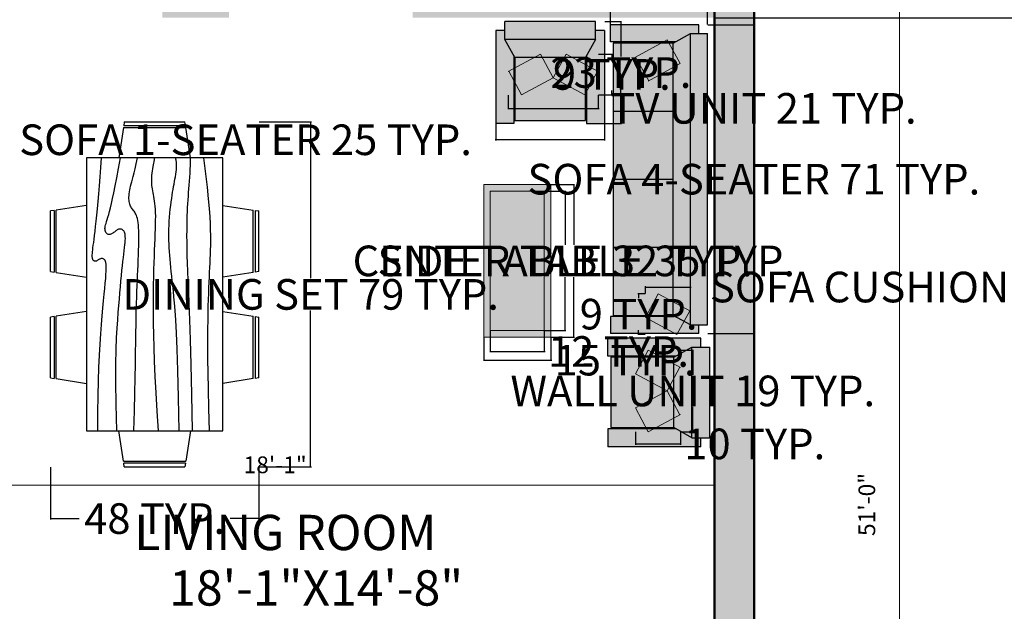
# Model space of a CAD drawing. Units: inches. Extents: x 1381 to 2246, y 1317 to 2168.
# Tile 7 of 15: x 1579 to 1804, y 1776 to 1911. Entities that reach past the tile are written whole.
import ezdxf

# ---------------------------------------------------------------- set-up
doc = ezdxf.new("R2010")
doc.units = ezdxf.units.IN
doc.header["$MEASUREMENT"] = 0
doc.layers.get('0').update_dxf_attribs({"color": 253})
for name, color, linetype, lineweight in [('A-ANNO-DIMS', 2, 'Continuous', 18), ('A-ANNO-TEXT', 7, 'Continuous', 18), ('A-AREA-IDEN', 3, 'Continuous', 25), ('A-FURN', 8, 'Continuous', 18), ('A-GLAZ', 4, 'Continuous', 25), ('A-WALL', 7, 'Continuous', 50)]:
    doc.layers.add(name, color=color, linetype=linetype, lineweight=lineweight)
doc.layers.add('furniture', color=250, linetype='Continuous')
doc.styles.get("Standard").update_dxf_attribs({"font": 'arial.ttf'})
doc.dimstyles.get("Standard").update_dxf_attribs({"dimtxt": 7, "dimasz": 0.18, "dimexe": 0.18, "dimexo": 0.0625, "dimgap": 0.09, "dimtad": 0, "dimtih": 1, "dimtoh": 1, "dimdec": 1, "dimzin": 0, "dimdsep": 46, "dimlunit": 3, "dimtxsty": 'Standard', "dimcen": 0.09, "dimadec": 0, "dimazin": 0, "dimtfac": 1, "dimtdec": 1, "dimtofl": 0, "dimtmove": 0, "dimatfit": 3, "dimfxl": 1, "dimtolj": 1, "dimtzin": 0, "dimarcsym": 0})

# ---------------------------------------------------------------- blocks, each defined once
blk = doc.blocks.new('Dining Set - 36 x 72 in.')
for p, q in [((-22.2343, 26.00059), (-23.4847, 17.99762)), ((-22.2304, 26), (-5.7608, 26)), ((-22, 27.5), (-22.1562, 26.50042)), ((-5.8416, 26.5), (-22.1534, 26.5)), ((-22, 27.5), (-6, 27.5)), ((-5.8437, 26.49966), (-6, 27.5)), ((-4.5152, 17.99762), (-5.7655, 25.99926)), ((5.7657, 26.00059), (4.5153, 17.99762)), ((5.7696, 26), (22.2392, 26)), ((6, 27.5), (5.8438, 26.50042)), ((22.1584, 26.5), (5.8466, 26.5)), ((6, 27.5), (22, 27.5)), ((22.1563, 26.49966), (22, 27.5)), ((23.4848, 17.99762), (22.2345, 25.99926)), ((36, 18), (-36, 18)), ((-36, 18), (-36, -18)), ((36, -18), (36, 18)), ((-45.5, 8), (-44.5004, 8.15617)), ((-45.5, 8), (-45.5, -8)), ((-44.5, -8.15843), (-44.5, 8.15338)), ((-44.0006, 8.23428), (-35.9976, 9.48474)), ((-44, 8.23041), (-44, -8.23915)), ((44.0006, 8.23428), (35.9976, 9.48474)), ((44, 8.23041), (44, -8.23915)), ((44.5, -8.15843), (44.5, 8.15338)), ((45.5, 8), (44.5005, 8.15617)), ((45.5, 8), (45.5, -8)), ((-44.4997, -8.15631), (-45.5, -8)), ((-35.9976, -9.48476), (-43.9993, -8.2345)), ((35.9976, -9.48476), (43.9993, -8.2345)), ((44.4997, -8.15631), (45.5, -8)), ((-36, -18), (36, -18)), ((-22.2343, -26.0006), (-23.4847, -17.99762)), ((-4.5152, -17.99762), (-5.7655, -25.99928)), ((5.7657, -26.0006), (4.5153, -17.99762)), ((23.4848, -17.99762), (22.2345, -25.99928)), ((-22.2304, -26), (-5.7608, -26)), ((-22, -27.5), (-22.1562, -26.50044)), ((-5.8416, -26.5), (-22.1534, -26.5)), ((-22, -27.5), (-6, -27.5)), ((-5.8437, -26.49967), (-6, -27.5)), ((5.7696, -26), (22.2392, -26)), ((6, -27.5), (5.8438, -26.50044)), ((22.1584, -26.5), (5.8466, -26.5)), ((6, -27.5), (22, -27.5)), ((22.1563, -26.49967), (22, -27.5))]:
    blk.add_line(p, q)
for points in [[(-36, 15), (-31.1772, 14.97754), (-26.8079, 14.91406), (-22.8538, 14.81543), (-19.276, 14.6875), (-16.0362, 14.53613), (-13.0957, 14.36718), (-10.4159, 14.18652), (-7.9583, 14), (-5.6904, 13.81315), (-3.6035, 13.63021), (-1.6954, 13.45508), (0.0365, 13.29166), (1.5945, 13.14388), (2.9811, 13.01562), (4.1988, 12.9108), (5.25, 12.83333), (6.1393, 12.78613), (6.8802, 12.76823), (7.4883, 12.77767), (7.9792, 12.8125), (8.3685, 12.87077), (8.6719, 12.95052), (8.9049, 13.0498), (9.0833, 13.16666), (9.2205, 13.29899), (9.3216, 13.44401), (9.3895, 13.59879), (9.4271, 13.76041), (9.4373, 13.92594), (9.4232, 14.09245), (9.3875, 14.257), (9.3333, 14.41666), (9.2638, 14.56917), (9.1836, 14.71484), (9.0975, 14.85465), (9.0104, 14.98958), (8.9272, 15.1206), (8.8529, 15.2487), (8.7922, 15.37483), (8.75, 15.5), (8.7305, 15.62467), (8.7344, 15.74739), (8.7617, 15.86621), (8.8125, 15.97916), (8.8867, 16.08431), (8.9844, 16.17968), (9.1055, 16.26334), (9.25, 16.33333), (9.4189, 16.38802), (9.6172, 16.42708), (9.8506, 16.45052), (10.125, 16.45833), (10.4463, 16.45052), (10.8203, 16.42708), (11.2529, 16.38802), (11.75, 16.33333), (12.3184, 16.26318), (12.9694, 16.17838), (13.7151, 16.07991), (14.5677, 15.96875), (15.5395, 15.84586), (16.6426, 15.71224), (17.8893, 15.56884), (19.2917, 15.41666), (20.859, 15.25667), (22.5879, 15.08984), (24.4721, 14.91715), (26.5052, 14.73958), (28.6809, 14.5581), (30.9929, 14.3737), (33.4347, 14.18733), (36, 14)], [(-36, 10), (-28.9766, 10.14274), (-23.1725, 10.20442), (-18.4241, 10.19775), (-14.5677, 10.13541), (-11.4399, 10.03011), (-8.877, 9.89453), (-6.7154, 9.74137), (-4.7917, 9.58333), (-2.9698, 9.43082), (-1.2246, 9.28515), (0.4415, 9.14534), (2.026, 9.01041), (3.5266, 8.87939), (4.9408, 8.7513), (6.266, 8.62516), (7.5, 8.5), (8.6411, 8.37549), (9.6914, 8.2539), (10.6538, 8.13818), (11.5312, 8.03125), (12.3267, 7.93603), (13.043, 7.85547), (13.6831, 7.79248), (14.25, 7.75), (14.7471, 7.7303), (15.1797, 7.73307), (15.5537, 7.75732), (15.875, 7.80208), (16.1494, 7.86637), (16.3828, 7.94922), (16.5811, 8.04964), (16.75, 8.16666), (16.8944, 8.29915), (17.0143, 8.44531), (17.1089, 8.60319), (17.1771, 8.77083), (17.218, 8.94629), (17.2305, 9.1276), (17.2137, 9.31282), (17.1667, 9.5), (17.0895, 9.6875), (16.987, 9.875), (16.8649, 10.0625), (16.7292, 10.25), (16.5856, 10.4375), (16.4401, 10.625), (16.2985, 10.8125), (16.1667, 11), (16.05, 11.18733), (15.9518, 11.3737), (15.8752, 11.5581), (15.8229, 11.73958), (15.798, 11.91715), (15.8034, 12.08984), (15.842, 12.25667), (15.9167, 12.41666), (16.0295, 12.56836), (16.1784, 12.70833), (16.3605, 12.83268), (16.5729, 12.9375), (16.8127, 13.01888), (17.0768, 13.07291), (17.3625, 13.0957), (17.6667, 13.08333), (17.9894, 13.03312), (18.3418, 12.94726), (18.7382, 12.82918), (19.1927, 12.68229), (19.7195, 12.51001), (20.3327, 12.31575), (21.0465, 12.10294), (21.875, 11.875), (22.8357, 11.63354), (23.959, 11.37304), (25.2786, 11.08618), (26.8282, 10.76562), (28.6414, 10.40405), (30.752, 9.99414), (33.1936, 9.52856), (36, 9)], [(-36, 5.5), (-30.7157, 5.3348), (-26.069, 5.20963), (-21.9946, 5.11767), (-18.4271, 5.05208), (-15.3009, 5.00602), (-12.5508, 4.97265), (-10.1112, 4.94515), (-7.9167, 4.91666), (-5.909, 4.88167), (-4.0586, 4.83984), (-2.3429, 4.79215), (-0.7396, 4.73958), (0.7739, 4.6831), (2.22, 4.6237), (3.6213, 4.56233), (5, 4.5), (6.373, 4.43782), (7.7344, 4.3776), (9.0723, 4.32129), (10.375, 4.27083), (11.6309, 4.22819), (12.8281, 4.19531), (13.9551, 4.17415), (15, 4.16666), (15.954, 4.17448), (16.819, 4.19791), (17.6001, 4.23698), (18.3021, 4.29166), (18.9299, 4.36198), (19.4883, 4.44791), (19.9823, 4.54948), (20.4167, 4.66666), (20.7969, 4.79899), (21.1302, 4.94401), (21.4245, 5.09879), (21.6875, 5.26041), (21.9271, 5.42594), (22.1511, 5.59245), (22.3672, 5.757), (22.5834, 5.91666), (22.8065, 6.06868), (23.0404, 6.21093), (23.2879, 6.34147), (23.5521, 6.45833), (23.8358, 6.55957), (24.142, 6.64323), (24.4735, 6.70735), (24.8334, 6.75), (25.2235, 6.76969), (25.642, 6.76692), (26.0858, 6.74267), (26.5521, 6.69791), (27.0379, 6.63362), (27.5404, 6.55078), (28.0565, 6.45036), (28.5834, 6.33333), (29.1242, 6.19987), (29.7071, 6.04687), (30.3661, 5.87044), (31.1354, 5.66666), (32.0493, 5.43164), (33.142, 5.16146), (34.4475, 4.85221), (36, 4.5)], [(-36, -1), (-30.7915, -0.6591), (-26.0195, -0.38216), (-21.6519, -0.16284), (-17.6563, 0.00521), (-14.0005, 0.12833), (-10.6523, 0.21289), (-7.5796, 0.26522), (-4.75, 0.29166), (-2.134, 0.29793), (0.2878, 0.28711), (2.5317, 0.26163), (4.6146, 0.22396), (6.5529, 0.17651), (8.3633, 0.12174), (10.0623, 0.06209), (11.6667, 0), (13.1899, -0.06201), (14.6341, -0.1211), (15.9982, -0.17432), (17.2813, -0.21875), (18.4823, -0.25147), (19.6003, -0.26953), (20.6343, -0.27002), (21.5834, -0.25), (22.4481, -0.20768), (23.2357, -0.14584), (23.9549, -0.06836), (24.6146, 0.02083), (25.2235, 0.11784), (25.7904, 0.21875), (26.3241, 0.31966), (26.8334, 0.41666), (27.3265, 0.50618), (27.8099, 0.58593), (28.2894, 0.65397), (28.7709, 0.70833), (29.2601, 0.74707), (29.763, 0.76823), (30.2855, 0.76985), (30.8334, 0.75), (31.4088, 0.70784), (31.9994, 0.64713), (32.589, 0.57275), (33.1615, 0.48958), (33.7008, 0.4025), (34.1908, 0.3164), (34.6153, 0.23616), (34.9584, 0.16666), (35.2099, 0.11165), (35.3848, 0.07031), (35.504, 0.04069), (35.5886, 0.02083), (35.6594, 0.00879), (35.7377, 0.0026), (35.8442, 0.00032), (36, 0)], [(-36, -6.5), (-27.1843, -6.31267), (-20.084, -6.1263), (-14.469, -5.9419), (-10.1094, -5.76042), (-6.7752, -5.58285), (-4.2363, -5.41016), (-2.2629, -5.24333), (-0.625, -5.08334), (0.8708, -4.93099), (2.2715, -4.78646), (3.5872, -4.64974), (4.8281, -4.52084), (6.0046, -4.39974), (7.127, -4.28646), (8.2053, -4.18099), (9.25, -4.08334), (10.2705, -3.99382), (11.2734, -3.91407), (12.2647, -3.84603), (13.25, -3.79167), (14.2354, -3.75293), (15.2266, -3.73177), (16.2295, -3.73015), (17.25, -3.75), (18.2912, -3.79248), (19.3451, -3.85547), (20.4009, -3.93604), (21.4479, -4.03125), (22.4754, -4.13819), (23.4727, -4.25391), (24.4289, -4.37549), (25.3334, -4.5), (26.1785, -4.62492), (26.9694, -4.74935), (27.7145, -4.87281), (28.4219, -4.99479), (29.1, -5.11483), (29.7572, -5.23242), (30.4016, -5.34709), (31.0417, -5.45834), (31.6837, -5.56437), (32.3262, -5.65821), (32.9658, -5.73153), (33.599, -5.77604), (34.2224, -5.78345), (34.8327, -5.74545), (35.4264, -5.65373), (36, -5.5)], [(-36, -10), (-26.4022, -9.81299), (-18.4675, -9.62891), (-11.9839, -9.45069), (-6.7396, -9.28125), (-2.5226, -9.12354), (0.8789, -8.98047), (3.6769, -8.85498), (6.0833, -8.75), (8.2767, -8.66765), (10.3021, -8.60677), (12.1712, -8.56543), (13.8958, -8.54167), (15.4876, -8.53353), (16.9583, -8.53907), (18.3197, -8.55632), (19.5834, -8.58334), (20.7616, -8.61841), (21.8685, -8.66081), (22.9188, -8.71004), (23.9271, -8.76563), (24.9081, -8.82707), (25.8763, -8.89388), (26.8465, -8.96558), (27.8334, -9.04167), (28.8474, -9.12118), (29.8828, -9.20117), (30.93, -9.27824), (31.9792, -9.34896), (33.0205, -9.40991), (34.0443, -9.45768), (35.0407, -9.48885), (36, -9.5)], [(-36, -14.5), (-30.0881, -14.33513), (-25.0332, -14.21224), (-20.7312, -14.12647), (-17.0781, -14.07292), (-13.97, -14.04671), (-11.3027, -14.04297), (-8.9724, -14.05681), (-6.875, -14.08334), (-4.9224, -14.11833), (-3.0905, -14.16016), (-1.3709, -14.20785), (0.2448, -14.26042), (1.7647, -14.3169), (3.1973, -14.3763), (4.5507, -14.43767), (5.8333, -14.5), (7.0554, -14.5621), (8.235, -14.62175), (9.3922, -14.67652), (10.5469, -14.72396), (11.7192, -14.76164), (12.929, -14.78711), (14.1965, -14.79794), (15.5417, -14.79167), (16.9933, -14.76424), (18.6152, -14.70508), (20.4804, -14.60197), (22.6615, -14.44271), (25.2312, -14.21509), (28.2624, -13.9069), (31.8277, -13.50594), (36, -13)]]:
    blk.add_lwpolyline(points)
blk = doc.blocks.new('dining area')
at = {"layer": 'furniture', "xscale": 0.6659924291999282, "yscale": 0.6659924291999282, "zscale": 0.6659924291999282, "rotation": 90}
blk.add_blockref('Dining Set - 36 x 72 in.', (-0.44, 20.51), dxfattribs=at)
blk = doc.blocks.new('FABRIC SOFA 4S')
at = {"layer": 'furniture'}
for p, q in [((3, 54), (34, 54)), ((3, 51), (3, 54)), ((34, 48), (34, 54)), ((0, -51), (0, 51)), ((6, 51), (0, 51)), ((6, -51), (6, 51)), ((12, 47.63), (6, 51)), ((11.14, 48), (34, 48)), ((33, 23.81), (12, 23.81)), ((33, 0), (12, 0)), ((33, -23.81), (12, -23.81)), ((6, -51), (12, -47.63)), ((11.54, -48), (34, -48)), ((34, -48), (34, -54)), ((6, -51), (0, -51)), ((3, -54), (3, -51)), ((3, -54), (34, -54))]:
    blk.add_line(p, q, dxfattribs=at)
blk.add_lwpolyline([(12, -47.63), (12, 47.63), (33, 47.63), (33, -47.63)], close=True, dxfattribs=at)
blk = doc.blocks.new('FABRIC SOFA 1S')
at = {"layer": 'furniture'}
for p, q in [((3, 18.12), (34, 18.12)), ((3, 15.12), (3, 18.12)), ((34, 12.12), (34, 18.12)), ((0, -15.12), (0, 15.12)), ((6, 15.12), (0, 15.12)), ((6, -15.12), (6, 15.12)), ((12, 11.75), (6, 15.12)), ((11.33, 12.12), (34, 12.12)), ((6, -15.12), (12, -11.75)), ((11.33, -12.12), (34, -12.12)), ((34, -12.12), (34, -18.12)), ((6, -15.12), (0, -15.12)), ((3, -18.12), (3, -15.12)), ((3, -18.12), (34, -18.12))]:
    blk.add_line(p, q, dxfattribs=at)
blk.add_lwpolyline([(12, -11.75), (12, 11.75), (33, 11.75), (33, -11.75)], close=True, dxfattribs=at)
blk = doc.blocks.new('TV-UNIT')
for p, q in [((0, 5.36), (7.38, 9.32)), ((7.38, 9.32), (10.3, 3.88)), ((13.22, 9.32), (10.3, 3.88)), ((20.6, 5.36), (13.22, 9.32)), ((3.07, 0), (0.15, 5.44)), ((17.53, 0), (20.45, 5.44)), ((10.3, 3.88), (3.07, 0)), ((10.3, 3.88), (17.53, 0))]:
    blk.add_line(p, q)
blk = doc.blocks.new('WALL-UNIT')
for p, q in [((2.92, 18.64), (0, 13.2)), ((10.3, 14.68), (2.92, 18.64)), ((7.23, 9.32), (10.15, 14.76)), ((0, 13.2), (7.23, 9.32)), ((0, 5.44), (7.23, 9.32)), ((7.23, 9.32), (10.15, 3.88)), ((2.92, 0), (0, 5.44)), ((10.3, 3.96), (2.92, 0))]:
    blk.add_line(p, q)
blk = doc.blocks.new('SOFA-CUSHION')
for p, q in [((2.92, 9.32), (0, 3.88)), ((10.3, 5.36), (2.92, 9.32)), ((7.23, 0), (10.15, 5.44)), ((0, 3.88), (7.23, 0))]:
    blk.add_line(p, q)
blk = doc.blocks.new('CENTER-TABLE')
for p, q in [((0, 0), (0, 34.91)), ((0, 34.91), (15.37, 34.91)), ((15.37, 34.91), (15.37, 0)), ((15.37, 0), (0, 0))]:
    blk.add_line(p, q)
blk = doc.blocks.new('SIDE-TABLE')
for p, q in [((0, 0), (0, 31.87)), ((0, 31.87), (12.34, 31.87)), ((12.34, 31.87), (12.34, 0)), ((12.34, 0), (0, 0))]:
    blk.add_line(p, q)
blk = doc.blocks.new('*D23')
at = {"layer": 'A-ANNO-DIMS', "color": 0, "lineweight": -2, "transparency": 16777216}
for p, q in [((1687.53, 1887.18), (1687.53, 1883.34)), ((1712.38, 1887.18), (1712.38, 1883.34)), ((1687.53, 1883.52), (1687.35, 1883.52)), ((1712.2, 1883.52), (1687.71, 1883.52))]:
    blk.add_line(p, q, dxfattribs=at)
at = {"layer": 'A-ANNO-DIMS', "color": 0, "transparency": 16777216}
for points in [[(1687.71, 1883.55), (1687.71, 1883.49), (1687.53, 1883.52)], [(1712.2, 1883.55), (1712.2, 1883.49), (1712.38, 1883.52)]]:
    blk.add_solid(points, dxfattribs=at)
at = {"layer": 'Defpoints', "color": 0, "transparency": 16777216}
for p in [(1687.53, 1887.25), (1712.38, 1887.25), (1687.53, 1883.52)]:
    blk.add_point(p, dxfattribs=at)
at = {"layer": 'A-ANNO-DIMS', "color": 0, "transparency": 16777216, "insert": (1630.3, 1883.52), "char_height": 7, "attachment_point": 5}
blk.add_mtext('\\A1;SOFA 1-SEATER 25 TYP.', dxfattribs=at)
blk = doc.blocks.new('*D24')
at = {"layer": 'A-ANNO-DIMS', "color": 0, "lineweight": -2, "transparency": 16777216}
for p, q in [((1712.44, 1910.55), (1716.29, 1910.55)), ((1716.11, 1910.37), (1716.11, 1902.57)), ((1716.11, 1887.43), (1716.11, 1895.23)), ((1712.44, 1887.25), (1716.29, 1887.25))]:
    blk.add_line(p, q, dxfattribs=at)
at = {"layer": 'A-ANNO-DIMS', "color": 0, "transparency": 16777216}
for points in [[(1716.08, 1910.37), (1716.14, 1910.37), (1716.11, 1910.55)], [(1716.08, 1887.43), (1716.14, 1887.43), (1716.11, 1887.25)]]:
    blk.add_solid(points, dxfattribs=at)
at = {"layer": 'Defpoints', "color": 0, "transparency": 16777216}
for p in [(1712.38, 1910.55), (1712.38, 1887.25), (1716.11, 1887.25)]:
    blk.add_point(p, dxfattribs=at)
at = {"layer": 'A-ANNO-DIMS', "color": 0, "transparency": 16777216, "insert": (1716.11, 1898.9), "char_height": 7, "attachment_point": 5}
blk.add_mtext('\\A1;23 TYP.', dxfattribs=at)
blk = doc.blocks.new('*D25')
at = {"layer": 'A-ANNO-DIMS', "color": 0, "lineweight": -2, "transparency": 16777216}
for p, q in [((1721.71, 1848.36), (1721.71, 1850.02)), ((1721.89, 1849.84), (1731.83, 1849.84)), ((1732.01, 1848.36), (1732.01, 1850.02)), ((1732.01, 1849.84), (1732.19, 1849.84))]:
    blk.add_line(p, q, dxfattribs=at)
at = {"layer": 'A-ANNO-DIMS', "color": 0, "transparency": 16777216}
for points in [[(1721.89, 1849.87), (1721.89, 1849.81), (1721.71, 1849.84)], [(1731.83, 1849.87), (1731.83, 1849.81), (1732.01, 1849.84)]]:
    blk.add_solid(points, dxfattribs=at)
at = {"layer": 'Defpoints', "color": 0, "transparency": 16777216}
for p in [(1721.71, 1848.3), (1732.01, 1849.84), (1732.01, 1848.3)]:
    blk.add_point(p, dxfattribs=at)
at = {"layer": 'A-ANNO-DIMS', "color": 0, "transparency": 16777216, "insert": (1787.87, 1849.84), "char_height": 7, "attachment_point": 5}
blk.add_mtext('\\A1;SOFA CUSHION 10 TYP.', dxfattribs=at)
blk = doc.blocks.new('*D26')
at = {"layer": 'A-ANNO-DIMS', "color": 0, "lineweight": -2, "transparency": 16777216}
for p, q in [((1721.65, 1848.3), (1719.98, 1848.3)), ((1720.16, 1848.12), (1720.16, 1847.3)), ((1720.16, 1839.16), (1720.16, 1839.97)), ((1721.65, 1838.98), (1719.98, 1838.98))]:
    blk.add_line(p, q, dxfattribs=at)
at = {"layer": 'A-ANNO-DIMS', "color": 0, "transparency": 16777216}
for points in [[(1720.13, 1848.12), (1720.19, 1848.12), (1720.16, 1848.3)], [(1720.13, 1839.16), (1720.19, 1839.16), (1720.16, 1838.98)]]:
    blk.add_solid(points, dxfattribs=at)
at = {"layer": 'Defpoints', "color": 0, "transparency": 16777216}
for p in [(1720.16, 1848.3), (1721.71, 1848.3), (1721.71, 1838.98)]:
    blk.add_point(p, dxfattribs=at)
at = {"layer": 'A-ANNO-DIMS', "color": 0, "transparency": 16777216, "insert": (1720.16, 1843.64), "char_height": 7, "attachment_point": 5}
blk.add_mtext('\\A1;9 TYP.', dxfattribs=at)
blk = doc.blocks.new('*D27')
at = {"layer": 'A-ANNO-DIMS', "color": 0, "lineweight": -2, "transparency": 16777216}
for p, q in [((1633.41, 1887.6), (1645.36, 1887.6)), ((1645.18, 1887.42), (1645.18, 1851.87)), ((1645.18, 1808.9), (1645.18, 1844.45)), ((1633.41, 1808.72), (1645.36, 1808.72))]:
    blk.add_line(p, q, dxfattribs=at)
at = {"layer": 'A-ANNO-DIMS', "color": 0, "transparency": 16777216}
for points in [[(1645.15, 1887.42), (1645.21, 1887.42), (1645.18, 1887.6)], [(1645.15, 1808.9), (1645.21, 1808.9), (1645.18, 1808.72)]]:
    blk.add_solid(points, dxfattribs=at)
at = {"layer": 'Defpoints', "color": 0, "transparency": 16777216}
for p in [(1633.35, 1887.6), (1645.18, 1887.6), (1633.35, 1808.72)]:
    blk.add_point(p, dxfattribs=at)
at = {"layer": 'A-ANNO-DIMS', "color": 0, "transparency": 16777216, "insert": (1645.18, 1848.16), "char_height": 7, "attachment_point": 5}
blk.add_mtext('\\A1;DINING SET 79 TYP.', dxfattribs=at)
blk = doc.blocks.new('*D28')
at = {"layer": 'A-ANNO-DIMS', "color": 0, "lineweight": -2, "transparency": 16777216}
for p, q in [((1585.67, 1808.66), (1585.67, 1796.71)), ((1633.35, 1808.66), (1633.35, 1796.71)), ((1585.85, 1796.89), (1592.24, 1796.89)), ((1633.17, 1796.89), (1626.78, 1796.89))]:
    blk.add_line(p, q, dxfattribs=at)
at = {"layer": 'A-ANNO-DIMS', "color": 0, "transparency": 16777216}
for points in [[(1585.85, 1796.92), (1585.85, 1796.86), (1585.67, 1796.89)], [(1633.17, 1796.92), (1633.17, 1796.86), (1633.35, 1796.89)]]:
    blk.add_solid(points, dxfattribs=at)
at = {"layer": 'Defpoints', "color": 0, "transparency": 16777216}
for p in [(1585.67, 1808.72), (1633.35, 1808.72), (1633.35, 1796.89)]:
    blk.add_point(p, dxfattribs=at)
at = {"layer": 'A-ANNO-DIMS', "color": 0, "transparency": 16777216, "insert": (1609.51, 1796.89), "char_height": 7, "attachment_point": 5}
blk.add_mtext('\\A1;48 TYP.', dxfattribs=at)
blk = doc.blocks.new('*D29')
at = {"layer": 'A-ANNO-DIMS', "color": 0, "lineweight": -2, "transparency": 16777216}
for p, q in [((1735.99, 1909.81), (1746.7, 1909.81)), ((1746.52, 1909.63), (1746.52, 1878.22)), ((1746.52, 1839.38), (1746.52, 1870.79)), ((1735.99, 1839.2), (1746.7, 1839.2))]:
    blk.add_line(p, q, dxfattribs=at)
at = {"layer": 'A-ANNO-DIMS', "color": 0, "transparency": 16777216}
for points in [[(1746.49, 1909.63), (1746.55, 1909.63), (1746.52, 1909.81)], [(1746.49, 1839.38), (1746.55, 1839.38), (1746.52, 1839.2)]]:
    blk.add_solid(points, dxfattribs=at)
at = {"layer": 'Defpoints', "color": 0, "transparency": 16777216}
for p in [(1735.93, 1909.81), (1746.52, 1909.81), (1735.93, 1839.2)]:
    blk.add_point(p, dxfattribs=at)
at = {"layer": 'A-ANNO-DIMS', "color": 0, "transparency": 16777216, "insert": (1746.52, 1874.51), "char_height": 7, "attachment_point": 5}
blk.add_mtext('\\A1;SOFA 4-SEATER 71 TYP.', dxfattribs=at)
blk = doc.blocks.new('*D30')
at = {"layer": 'A-ANNO-DIMS', "color": 0, "lineweight": -2, "transparency": 16777216}
for p, q in [((1713.7, 1920.4), (1713.52, 1920.4)), ((1713.7, 1909.87), (1713.7, 1920.58)), ((1735.75, 1920.4), (1713.88, 1920.4)), ((1735.93, 1909.87), (1735.93, 1920.58))]:
    blk.add_line(p, q, dxfattribs=at)
at = {"layer": 'A-ANNO-DIMS', "color": 0, "transparency": 16777216}
for points in [[(1713.88, 1920.43), (1713.88, 1920.37), (1713.7, 1920.4)], [(1735.75, 1920.43), (1735.75, 1920.37), (1735.93, 1920.4)]]:
    blk.add_solid(points, dxfattribs=at)
at = {"layer": 'Defpoints', "color": 0, "transparency": 16777216}
for p in [(1713.7, 1920.4), (1713.7, 1909.81), (1735.93, 1909.81)]:
    blk.add_point(p, dxfattribs=at)
at = {"layer": 'A-ANNO-DIMS', "color": 0, "transparency": 16777216, "insert": (1696.34, 1920.4), "char_height": 7, "attachment_point": 5}
blk.add_mtext('\\A1;22 TYP.', dxfattribs=at)
blk = doc.blocks.new('*D37')
at = {"layer": 'A-ANNO-DIMS', "color": 0, "lineweight": -2, "transparency": 16777216}
for p, q in [((1690.35, 1893.74), (1690.35, 1890.53)), ((1710.95, 1893.74), (1710.95, 1890.53)), ((1690.53, 1890.71), (1710.77, 1890.71)), ((1710.95, 1890.71), (1711.13, 1890.71))]:
    blk.add_line(p, q, dxfattribs=at)
at = {"layer": 'A-ANNO-DIMS', "color": 0, "transparency": 16777216}
for points in [[(1690.53, 1890.74), (1690.53, 1890.68), (1690.35, 1890.71)], [(1710.77, 1890.74), (1710.77, 1890.68), (1710.95, 1890.71)]]:
    blk.add_solid(points, dxfattribs=at)
at = {"layer": 'Defpoints', "color": 0, "transparency": 16777216}
for p in [(1690.35, 1893.8), (1710.95, 1893.8), (1710.95, 1890.71)]:
    blk.add_point(p, dxfattribs=at)
at = {"layer": 'A-ANNO-DIMS', "color": 0, "transparency": 16777216, "insert": (1748.72, 1890.71), "char_height": 7, "attachment_point": 5}
blk.add_mtext('\\A1;TV UNIT 21 TYP.', dxfattribs=at)
blk = doc.blocks.new('*D38')
at = {"layer": 'A-ANNO-DIMS', "color": 0, "lineweight": -2, "transparency": 16777216}
for p, q in [((1711.02, 1903.12), (1714.22, 1903.12)), ((1714.04, 1902.94), (1714.04, 1902.12)), ((1711.02, 1893.8), (1714.22, 1893.8)), ((1714.04, 1893.98), (1714.04, 1894.79))]:
    blk.add_line(p, q, dxfattribs=at)
at = {"layer": 'A-ANNO-DIMS', "color": 0, "transparency": 16777216}
for points in [[(1714.01, 1902.94), (1714.07, 1902.94), (1714.04, 1903.12)], [(1714.01, 1893.98), (1714.07, 1893.98), (1714.04, 1893.8)]]:
    blk.add_solid(points, dxfattribs=at)
at = {"layer": 'Defpoints', "color": 0, "transparency": 16777216}
for p in [(1710.95, 1903.12), (1714.04, 1903.12), (1710.95, 1893.8)]:
    blk.add_point(p, dxfattribs=at)
at = {"layer": 'A-ANNO-DIMS', "color": 0, "transparency": 16777216, "insert": (1714.04, 1898.46), "char_height": 7, "attachment_point": 5}
blk.add_mtext('\\A1;9 TYP.', dxfattribs=at)
blk = doc.blocks.new('*D39')
at = {"layer": 'A-ANNO-DIMS', "color": 0, "lineweight": -2, "transparency": 16777216}
for p, q in [((1729.81, 1835.4), (1732.72, 1835.4)), ((1732.54, 1835.22), (1732.54, 1829.75)), ((1732.54, 1816.94), (1732.54, 1822.42)), ((1729.81, 1816.76), (1732.72, 1816.76))]:
    blk.add_line(p, q, dxfattribs=at)
at = {"layer": 'A-ANNO-DIMS', "color": 0, "transparency": 16777216}
for points in [[(1732.51, 1835.22), (1732.57, 1835.22), (1732.54, 1835.4)], [(1732.51, 1816.94), (1732.57, 1816.94), (1732.54, 1816.76)]]:
    blk.add_solid(points, dxfattribs=at)
at = {"layer": 'Defpoints', "color": 0, "transparency": 16777216}
for p in [(1729.74, 1835.4), (1732.54, 1835.4), (1729.74, 1816.76)]:
    blk.add_point(p, dxfattribs=at)
at = {"layer": 'A-ANNO-DIMS', "color": 0, "transparency": 16777216, "insert": (1732.54, 1826.08), "char_height": 7, "attachment_point": 5}
blk.add_mtext('\\A1;WALL UNIT 19 TYP.', dxfattribs=at)
blk = doc.blocks.new('*D40')
at = {"layer": 'A-ANNO-DIMS', "color": 0, "lineweight": -2, "transparency": 16777216}
for p, q in [((1719.44, 1816.7), (1719.44, 1813.79)), ((1729.74, 1816.7), (1729.74, 1813.79)), ((1719.62, 1813.97), (1729.56, 1813.97)), ((1729.74, 1813.97), (1729.92, 1813.97))]:
    blk.add_line(p, q, dxfattribs=at)
at = {"layer": 'A-ANNO-DIMS', "color": 0, "transparency": 16777216}
for points in [[(1719.62, 1814), (1719.62, 1813.94), (1719.44, 1813.97)], [(1729.56, 1814), (1729.56, 1813.94), (1729.74, 1813.97)]]:
    blk.add_solid(points, dxfattribs=at)
at = {"layer": 'Defpoints', "color": 0, "transparency": 16777216}
for p in [(1719.44, 1816.76), (1729.74, 1816.76), (1729.74, 1813.97)]:
    blk.add_point(p, dxfattribs=at)
at = {"layer": 'A-ANNO-DIMS', "color": 0, "transparency": 16777216, "insert": (1746.72, 1813.97), "char_height": 7, "attachment_point": 5}
blk.add_mtext('\\A1;10 TYP.', dxfattribs=at)
blk = doc.blocks.new('*D43')
at = {"layer": 'A-ANNO-DIMS', "color": 0, "lineweight": -2, "transparency": 16777216}
for p, q in [((1700.18, 1873.27), (1705.53, 1873.27)), ((1705.35, 1873.09), (1705.35, 1859.53)), ((1705.35, 1838.54), (1705.35, 1852.1)), ((1700.18, 1838.36), (1705.53, 1838.36))]:
    blk.add_line(p, q, dxfattribs=at)
at = {"layer": 'A-ANNO-DIMS', "color": 0, "transparency": 16777216}
for points in [[(1705.32, 1873.09), (1705.38, 1873.09), (1705.35, 1873.27)], [(1705.32, 1838.54), (1705.38, 1838.54), (1705.35, 1838.36)]]:
    blk.add_solid(points, dxfattribs=at)
at = {"layer": 'Defpoints', "color": 0, "transparency": 16777216}
for p in [(1700.11, 1873.27), (1705.35, 1873.27), (1700.11, 1838.36)]:
    blk.add_point(p, dxfattribs=at)
at = {"layer": 'A-ANNO-DIMS', "color": 0, "transparency": 16777216, "insert": (1705.35, 1855.82), "char_height": 7, "attachment_point": 5}
blk.add_mtext('\\A1;CENTER TABLE 35 TYP.', dxfattribs=at)
blk = doc.blocks.new('*D44')
at = {"layer": 'A-ANNO-DIMS', "color": 0, "lineweight": -2, "transparency": 16777216}
for p, q in [((1684.74, 1838.3), (1684.74, 1832.94)), ((1700.11, 1838.3), (1700.11, 1832.94)), ((1684.92, 1833.12), (1699.93, 1833.12)), ((1700.11, 1833.12), (1700.29, 1833.12))]:
    blk.add_line(p, q, dxfattribs=at)
at = {"layer": 'A-ANNO-DIMS', "color": 0, "transparency": 16777216}
for points in [[(1684.92, 1833.15), (1684.92, 1833.09), (1684.74, 1833.12)], [(1699.93, 1833.15), (1699.93, 1833.09), (1700.11, 1833.12)]]:
    blk.add_solid(points, dxfattribs=at)
at = {"layer": 'Defpoints', "color": 0, "transparency": 16777216}
for p in [(1684.74, 1838.36), (1700.11, 1838.36), (1700.11, 1833.12)]:
    blk.add_point(p, dxfattribs=at)
at = {"layer": 'A-ANNO-DIMS', "color": 0, "transparency": 16777216, "insert": (1717.09, 1833.12), "char_height": 7, "attachment_point": 5}
blk.add_mtext('\\A1;15 TYP.', dxfattribs=at)
blk = doc.blocks.new('*D45')
at = {"layer": 'A-ANNO-DIMS', "color": 0, "lineweight": -2, "transparency": 16777216}
for p, q in [((1698.66, 1871.75), (1703.55, 1871.75)), ((1703.37, 1871.57), (1703.37, 1859.53)), ((1703.37, 1840.06), (1703.37, 1852.1)), ((1698.66, 1839.88), (1703.55, 1839.88))]:
    blk.add_line(p, q, dxfattribs=at)
at = {"layer": 'A-ANNO-DIMS', "color": 0, "transparency": 16777216}
for points in [[(1703.34, 1871.57), (1703.4, 1871.57), (1703.37, 1871.75)], [(1703.34, 1840.06), (1703.4, 1840.06), (1703.37, 1839.88)]]:
    blk.add_solid(points, dxfattribs=at)
at = {"layer": 'Defpoints', "color": 0, "transparency": 16777216}
for p in [(1698.59, 1871.75), (1703.37, 1871.75), (1698.59, 1839.88)]:
    blk.add_point(p, dxfattribs=at)
at = {"layer": 'A-ANNO-DIMS', "color": 0, "transparency": 16777216, "insert": (1703.37, 1855.82), "char_height": 7, "attachment_point": 5}
blk.add_mtext('\\A1;SIDE TABLE 32 TYP.', dxfattribs=at)
blk = doc.blocks.new('*D46')
at = {"layer": 'A-ANNO-DIMS', "color": 0, "lineweight": -2, "transparency": 16777216}
for p, q in [((1686.26, 1839.82), (1686.26, 1834.92)), ((1698.59, 1839.82), (1698.59, 1834.92)), ((1686.44, 1835.1), (1698.41, 1835.1)), ((1698.59, 1835.1), (1698.77, 1835.1))]:
    blk.add_line(p, q, dxfattribs=at)
at = {"layer": 'A-ANNO-DIMS', "color": 0, "transparency": 16777216}
for points in [[(1686.44, 1835.13), (1686.44, 1835.07), (1686.26, 1835.1)], [(1698.41, 1835.13), (1698.41, 1835.07), (1698.59, 1835.1)]]:
    blk.add_solid(points, dxfattribs=at)
at = {"layer": 'Defpoints', "color": 0, "transparency": 16777216}
for p in [(1686.26, 1839.88), (1698.59, 1839.88), (1698.59, 1835.1)]:
    blk.add_point(p, dxfattribs=at)
at = {"layer": 'A-ANNO-DIMS', "color": 0, "transparency": 16777216, "insert": (1715.57, 1835.1), "char_height": 7, "attachment_point": 5}
blk.add_mtext('\\A1;12 TYP.', dxfattribs=at)
blk = doc.blocks.new('*D61')
at = {"layer": 'A-ANNO-DIMS', "color": 0, "lineweight": -2, "transparency": 16777216}
for p, q in [((1737.61, 1911.42), (1818.27, 1911.42)), ((1818.09, 1911.24), (1818.09, 1808.63)), ((1818.09, 1698.7), (1818.09, 1801.3)), ((1737.61, 1698.52), (1818.27, 1698.52))]:
    blk.add_line(p, q, dxfattribs=at)
at = {"layer": 'A-ANNO-DIMS', "color": 0, "transparency": 16777216}
for points in [[(1818.06, 1911.24), (1818.12, 1911.24), (1818.09, 1911.42)], [(1818.06, 1698.7), (1818.12, 1698.7), (1818.09, 1698.52)]]:
    blk.add_solid(points, dxfattribs=at)
at = {"layer": 'Defpoints', "color": 0, "transparency": 16777216}
for p in [(1737.55, 1911.42), (1818.09, 1911.42), (1737.55, 1698.52)]:
    blk.add_point(p, dxfattribs=at)
at = {"layer": 'A-ANNO-DIMS', "color": 0, "transparency": 16777216, "insert": (1818.09, 1804.97), "char_height": 7, "attachment_point": 5}
blk.add_mtext('\\A1;212.9', dxfattribs=at)

msp = doc.modelspace()

# ---------------------------------------------------------------- hatches: boundary and pattern name
at = {"layer": 'A-FURN'}
h = msp.add_hatch(color=256, dxfattribs=at)
h.dxf.hatch_style = 1
h.paths.add_polyline_path([(1708.0086, 1902.3282), (1691.8983, 1902.3282), (1691.8983, 1887.9317), (1708.0086, 1887.9317)])
h.paths.add_polyline_path([(1710.3223, 1906.4414), (1689.5846, 1906.4414), (1691.8983, 1902.3282), (1708.0086, 1902.3282)])
h.paths.add_polyline_path([(1710.3223, 1910.5547), (1689.5846, 1910.5547), (1689.5846, 1906.4414), (1710.3223, 1906.4414)])
h.paths.add_polyline_path([(1691.6412, 1902.7852), (1689.5846, 1906.4414), (1689.5846, 1908.4981), (1687.5279, 1908.4981), (1687.5279, 1887.2462), (1691.6412, 1887.2462)])
h.paths.add_polyline_path([(1712.3789, 1908.4981), (1710.3223, 1908.4981), (1710.3223, 1906.4414), (1708.2657, 1902.7852), (1708.2657, 1887.2462), (1712.3789, 1887.2462)])
h = msp.add_hatch(color=256, dxfattribs=at)
h.dxf.hatch_style = 1
h.paths.add_polyline_path([(1732.0082, 1907.8492), (1733.9696, 1907.8492), (1733.9696, 1909.8106), (1713.702, 1909.8106), (1713.702, 1905.8878), (1728.5213, 1905.8878)])
h.paths.add_polyline_path([(1728.0854, 1905.6427), (1714.3558, 1905.6427), (1714.3558, 1890.0742), (1728.0854, 1890.0742)])
h.paths.add_polyline_path([(1728.0854, 1890.0742), (1714.3558, 1890.0742), (1714.3558, 1874.5057), (1728.0854, 1874.5057)])
h.paths.add_polyline_path([(1728.0854, 1874.5057), (1714.3558, 1874.5057), (1714.3558, 1858.9372), (1728.0854, 1858.9372)])
h = msp.add_hatch(color=256, dxfattribs=at)
h.dxf.hatch_style = 1
h.paths.add_polyline_path([(1735.931, 1907.8492), (1732.0082, 1907.8492), (1732.0082, 1841.1622), (1735.931, 1841.1622)])
h.paths.add_polyline_path([(1732.0082, 1907.8492), (1728.0854, 1905.6427), (1728.0854, 1843.3688), (1732.0082, 1841.1622)])
h.paths.add_polyline_path([(1728.0854, 1858.9372), (1714.3558, 1858.9372), (1714.3558, 1843.3688), (1728.0854, 1843.3688)])
h.paths.add_polyline_path([(1732.0082, 1841.1622), (1728.5213, 1843.1236), (1713.702, 1843.1236), (1713.702, 1839.2008), (1733.9696, 1839.2008), (1733.9696, 1841.1622)])
h = msp.add_hatch(color=256, dxfattribs=at)
h.dxf.hatch_style = 1
h.paths.add_polyline_path([(1722.3751, 1897.028), (1729.6072, 1900.9083), (1726.6895, 1906.3465), (1719.4573, 1902.4662)])
h = msp.add_hatch(color=256, dxfattribs=at)
h.dxf.hatch_style = 1
h.paths.add_polyline_path([(1697.7355, 1903.1174), (1690.5034, 1899.2371), (1693.4211, 1893.799), (1700.6533, 1897.6793)])
h = msp.add_hatch(color=256, dxfattribs=at)
h.dxf.hatch_style = 1
h.paths.add_polyline_path([(1703.571, 1903.1174), (1710.8032, 1899.2371), (1707.8855, 1893.799), (1700.6533, 1897.6793)])
h = msp.add_hatch(color=256, dxfattribs=at)
h.dxf.hatch_style = 1
h.paths.add_polyline_path([(1700.113, 1873.2707), (1684.7389, 1873.2707), (1684.7389, 1838.3593), (1700.113, 1838.3593)])
h.paths.add_polyline_path([(1686.2582, 1871.7514), (1698.5937, 1871.7514), (1698.5937, 1839.8786), (1686.2582, 1839.8786)], flags=16)
h = msp.add_hatch(color=256, dxfattribs=at)
h.dxf.hatch_style = 1
h.paths.add_polyline_path([(1698.5937, 1871.7514), (1686.2582, 1871.7514), (1686.2582, 1839.8786), (1698.5937, 1839.8786)])
h = msp.add_hatch(color=256, dxfattribs=at)
h.dxf.hatch_style = 1
h.paths.add_polyline_path([(1724.6258, 1848.2968), (1731.858, 1844.4165), (1728.9403, 1838.9783), (1721.7081, 1842.8586)])
h = msp.add_hatch(color=256, dxfattribs=at)
h.dxf.hatch_style = 1
h.paths.add_polyline_path([(1734.3967, 1838.1626), (1713.1448, 1838.1626), (1713.1448, 1834.0493), (1728.6839, 1834.0493), (1732.3401, 1836.106), (1734.3967, 1836.106)])
h.paths.add_polyline_path([(1728.2268, 1833.7922), (1713.8304, 1833.7922), (1713.8304, 1817.6819), (1728.2268, 1817.6819)])
h.paths.add_polyline_path([(1734.3967, 1815.3682), (1732.3401, 1815.3682), (1728.6839, 1817.4249), (1713.1448, 1817.4249), (1713.1448, 1813.3116), (1734.3967, 1813.3116)])
h.paths.add_polyline_path([(1732.3401, 1836.106), (1728.2268, 1833.7922), (1728.2268, 1817.6819), (1732.3401, 1815.3682)])
h.paths.add_polyline_path([(1736.4534, 1836.106), (1732.3401, 1836.106), (1732.3401, 1815.3682), (1736.4534, 1815.3682)])
h = msp.add_hatch(color=256, dxfattribs=at)
h.dxf.hatch_style = 1
h.paths.add_polyline_path([(1722.3619, 1835.4011), (1729.594, 1831.5208), (1726.6763, 1826.0827), (1719.4441, 1829.963)])
h = msp.add_hatch(color=256, dxfattribs=at)
h.dxf.hatch_style = 1
h.paths.add_polyline_path([(1722.3619, 1816.7642), (1729.594, 1820.6445), (1726.6763, 1826.0827), (1719.4441, 1822.2024)])
at = {"layer": 'A-GLAZ'}
h = msp.add_hatch(color=256, dxfattribs=at)
h.dxf.hatch_style = 1
h.paths.add_polyline_path([(1456.051, 2083.9163), (1737.551, 2083.9163), (1737.551, 1677.4163), (1732.8596, 1677.4163), (1732.8596, 1672.9163), (1737.551, 1672.9163), (1737.551, 1471.9163), (1746.551, 1471.9163), (1746.551, 2092.9163), (1447.051, 2092.9163), (1447.051, 2083.9163), (1447.051, 1471.9163), (1488.6632, 1471.9163), (1488.6632, 1480.9163), (1456.051, 1480.9163), (1456.051, 1710.4163), (1517.1194, 1710.4163), (1517.1194, 1714.9163), (1491.551, 1714.9163), (1491.551, 1729.193), (1487.051, 1729.193), (1487.051, 1714.9163), (1456.051, 1714.9163)])
h.paths.add_polyline_path([(1622.551, 2035.4163), (1625.0954, 2035.4163), (1625.0954, 2039.9163), (1618.051, 2039.9163), (1618.051, 1915.9163), (1611.2353, 1915.9163), (1611.2353, 1911.4163), (1626.5102, 1911.4163), (1626.5102, 1915.9163), (1622.551, 1915.9163)], flags=17)
h.paths.add_polyline_path([(1737.551, 1915.9163), (1668.5102, 1915.9163), (1668.5102, 1911.4163), (1737.551, 1911.4163)], flags=17)
h.paths.add_polyline_path([(1682.2831, 2039.9163), (1655.8191, 2039.9163), (1655.8191, 2035.4163), (1682.2831, 2035.4163)], flags=17)
h.paths.add_polyline_path([(1737.551, 2039.9163), (1725.9636, 2039.9163), (1725.9636, 2035.4163), (1737.551, 2035.4163)], flags=17)
h.paths.add_polyline_path([(1684.2508, 1711.4667), (1740.8192, 1711.4667), (1740.8192, 1723.8346), (1684.2508, 1723.8346)], flags=25)

# ---------------------------------------------------------------- linework, layer by layer
at = {"layer": 'A-ANNO-DIMS'}
for p, q in [((1779.8404, 2092.9163), (1779.8404, 1471.9163)), ((1520.551, 1804.4959), (1737.551, 1804.4959))]:
    msp.add_line(p, q, dxfattribs=at)
at = {"layer": 'A-WALL'}
for p, q in [((1746.551, 2092.9163), (1746.551, 1471.9163)), ((1737.551, 2083.9163), (1737.551, 1677.4163))]:
    msp.add_line(p, q, dxfattribs=at)

# ---------------------------------------------------------------- block references
at = {"layer": 'A-FURN'}
for name, p, xscale, yscale, zscale, rotation in [('FABRIC SOFA 1S', (1699.9534, 1910.5547), -0.685544738852578, 0.685544738852578, 0.685544738852578, 90), ('FABRIC SOFA 4S', (1735.931, 1874.5057), -0.6537939928824033, 0.6537939928824033, 0.6537939928824033, 359.9999999998932)]:
    msp.add_blockref(name, p, dxfattribs=dict(at, xscale=xscale, yscale=yscale, zscale=zscale, rotation=rotation))
at = {"layer": 'A-FURN', "rotation": 237.2649470423719}
msp.add_blockref('SOFA-CUSHION', (1723.3945, 1908.4964), dxfattribs=at)
at = {"layer": 'A-FURN'}
for name, p in [('TV-UNIT', (1690.353, 1893.799)), ('CENTER-TABLE', (1684.739, 1838.359)), ('SIDE-TABLE', (1686.258, 1839.879)), ('SOFA-CUSHION', (1721.708, 1838.978)), ('WALL-UNIT', (1719.444, 1816.764))]:
    msp.add_blockref(name, p, dxfattribs=at)
for name, p, xscale, yscale, zscale in [('dining area', (1610.0826, 1821.4677), 1.301533394022331, 1.301533394022331, 1.301533394022331), ('FABRIC SOFA 1S', (1736.4534, 1825.7371), -0.685544738852578, 0.685544738852578, 0.685544738852578)]:
    msp.add_blockref(name, p, dxfattribs=dict(at, xscale=xscale, yscale=yscale, zscale=zscale))

# ---------------------------------------------------------------- texts
at = {"layer": 'A-ANNO-TEXT'}
msp.add_text('18\'-1"', height=3.83139, dxfattribs=at).set_placement((1629.828, 1807.2715))
msp.add_text('51\'-0"', height=3.83139, rotation=90, dxfattribs=at).set_placement((1774.2617, 1792.8891))
at = {"layer": 'A-AREA-IDEN'}
for s, p in [('LIVING ROOM', (1604.8492, 1789.6702)), ('18\'-1"X14\'-8"', (1612.8376, 1776.9826))]:
    msp.add_text(s, height=8.074511, dxfattribs=at).set_placement(p)

# ---------------------------------------------------------------- dimensions: what is measured, and where the dimension line sits
at = {"layer": 'A-ANNO-DIMS'}
for base, p1, p2, angle, text, picture, middle in [((1713.702, 1920.4021), (1735.931, 1909.8106), (1713.702, 1909.8106), 180, '<> TYP.', '*D30', (1696.3354, 1920.4021)), ((1746.5224, 1909.8106), (1735.931, 1839.2008), (1735.931, 1909.8106), 90, 'SOFA 4-SEATER <> TYP.', '*D29', (1746.5224, 1874.5057)), ((1716.1066, 1887.2462), (1712.3789, 1910.5547), (1712.3789, 1887.2462), 270, '<> TYP.', '*D24', (1716.1066, 1898.9005)), ((1714.0434, 1903.1174), (1710.9534, 1893.799), (1710.9534, 1903.1174), 90, '<> TYP.', '*D38', (1714.0434, 1898.4582)), ((1687.5279, 1883.5185), (1712.3789, 1887.2462), (1687.5279, 1887.2462), 180, 'SOFA 1-SEATER <> TYP.', '*D23', (1630.2982, 1883.5185)), ((1645.1805, 1887.598), (1633.3486, 1808.7182), (1633.3486, 1887.598), 90, 'DINING SET <> TYP.', '*D27', (1645.1805, 1848.1581)), ((1705.3497, 1873.2707), (1700.113, 1838.3593), (1700.113, 1873.2707), 90, 'CENTER TABLE <> TYP.', '*D43', (1705.3497, 1855.815)), ((1703.3747, 1871.7514), (1698.5937, 1839.8786), (1698.5937, 1871.7514), 90, 'SIDE TABLE <> TYP.', '*D45', (1703.3747, 1855.815)), ((1720.1631, 1848.2968), (1721.7081, 1838.9783), (1721.7081, 1848.2968), 90, '<> TYP.', '*D26', (1720.1631, 1843.6376)), ((1732.5398, 1835.4011), (1729.7442, 1816.7642), (1729.7442, 1835.4011), 90, 'WALL UNIT <> TYP.', '*D39', (1732.5398, 1826.0827))]:
    dim = msp.add_linear_dim(base=base, p1=p1, p2=p2, angle=angle, text=text, dimstyle='Standard', override={"dimdec": 0, "dimrnd": 0, "dimzin": 0, "dimlunit": 2}, dxfattribs=at)
    dim.commit()
    dim.dimension.update_dxf_attribs({"geometry": picture, "text_midpoint": middle})
for base, p1, p2, text, picture, middle in [((1710.9534, 1890.7089), (1690.3532, 1893.799), (1710.9534, 1893.799), 'TV UNIT <> TYP.', '*D37', (1748.7207, 1890.7089)), ((1732.0082, 1849.8418), (1721.7081, 1848.2968), (1732.0082, 1848.2968), 'SOFA CUSHION <> TYP.', '*D25', (1787.8747, 1849.8418)), ((1698.5937, 1835.0977), (1686.2582, 1839.8786), (1698.5937, 1839.8786), '<> TYP.', '*D46', (1715.5711, 1835.0977)), ((1700.113, 1833.1226), (1684.7389, 1838.3593), (1700.113, 1838.3593), '<> TYP.', '*D44', (1717.0904, 1833.1226)), ((1729.7442, 1813.9687), (1719.4441, 1816.7642), (1729.7442, 1816.7642), '<> TYP.', '*D40', (1746.7216, 1813.9687)), ((1633.3486, 1796.8862), (1585.6739, 1808.7182), (1633.3486, 1808.7182), '<> TYP.', '*D28', (1609.5112, 1796.8862))]:
    dim = msp.add_linear_dim(base=base, p1=p1, p2=p2, text=text, dimstyle='Standard', override={"dimdec": 0, "dimrnd": 0, "dimzin": 0, "dimlunit": 2}, dxfattribs=at)
    dim.commit()
    dim.dimension.update_dxf_attribs({"geometry": picture, "text_midpoint": middle})
dim = msp.add_linear_dim(base=(1818.0904, 1911.4163), p1=(1737.551, 1698.5169), p2=(1737.551, 1911.4163), angle=90, dimstyle='Standard', override={"dimdec": 1, "dimlfac": 1, "dimrnd": 0, "dimzin": 0, "dimdsep": 46, "dimlunit": 2}, dxfattribs=at)
dim.commit()
dim.dimension.update_dxf_attribs({"geometry": '*D61', "text_midpoint": (1818.0904, 1804.9666)})

doc.saveas('drawing.dxf')
